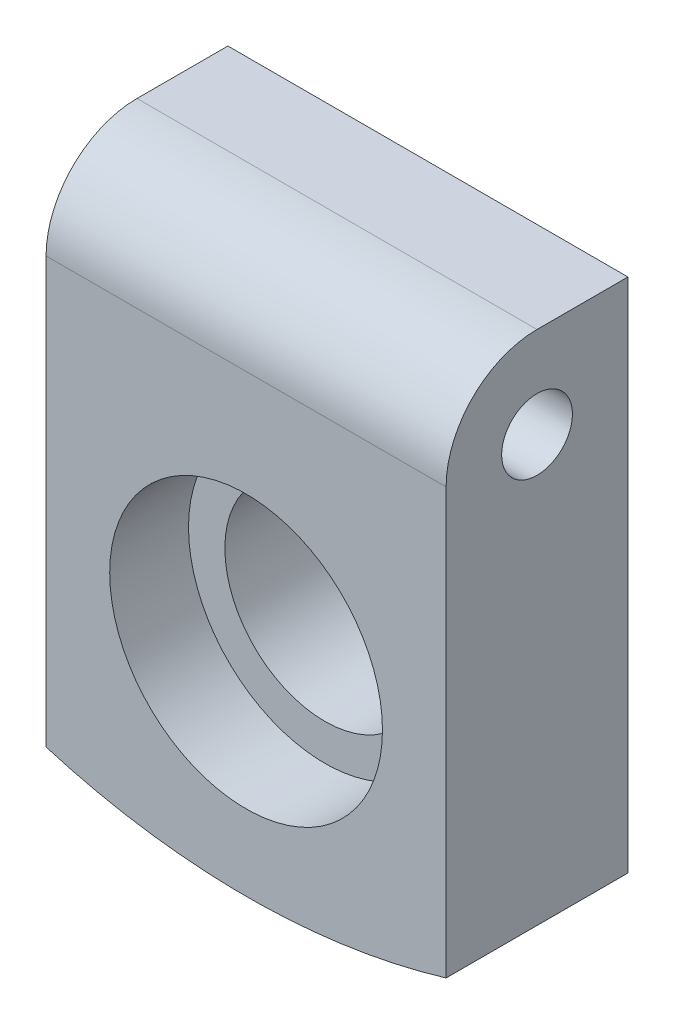
ISO-10303-21;
HEADER;
FILE_DESCRIPTION(('STEP AP214'),'2;1');
FILE_NAME('part.step','',(''),(''),'','','');
FILE_SCHEMA(('AUTOMOTIVE_DESIGN { 1 0 10303 214 1 1 1 1 }'));
ENDSEC;
DATA;
#1=APPLICATION_CONTEXT('core data for automotive mechanical design processes');
#2=APPLICATION_PROTOCOL_DEFINITION('international standard','automotive_design',2000,#1);
#3=PRODUCT_CONTEXT('',#1,'mechanical');
#4=PRODUCT('Part','Part','',(#3));
#5=PRODUCT_RELATED_PRODUCT_CATEGORY('part','',(#4));
#6=PRODUCT_DEFINITION_FORMATION('','',#4);
#7=PRODUCT_DEFINITION_CONTEXT('part definition',#1,'design');
#8=PRODUCT_DEFINITION('design','',#6,#7);
#9=PRODUCT_DEFINITION_SHAPE('','',#8);
#10=(LENGTH_UNIT() NAMED_UNIT(*) SI_UNIT(.MILLI.,.METRE.));
#11=(NAMED_UNIT(*) PLANE_ANGLE_UNIT() SI_UNIT($,.RADIAN.));
#12=(NAMED_UNIT(*) SI_UNIT($,.STERADIAN.) SOLID_ANGLE_UNIT());
#13=UNCERTAINTY_MEASURE_WITH_UNIT(LENGTH_MEASURE(1.E-05),#10,'distance_accuracy_value','');
#14=(GEOMETRIC_REPRESENTATION_CONTEXT(3) GLOBAL_UNCERTAINTY_ASSIGNED_CONTEXT((#13)) GLOBAL_UNIT_ASSIGNED_CONTEXT((#10,
#11,#12)) REPRESENTATION_CONTEXT('',''));
#15=CARTESIAN_POINT('',(0.,0.,0.));
#16=DIRECTION('',(0.,0.,1.));
#17=DIRECTION('',(1.,0.,0.));
#18=AXIS2_PLACEMENT_3D('',#15,#16,#17);
#19=CARTESIAN_POINT('',(0.,0.,15.));
#20=DIRECTION('',(0.,0.,-1.));
#21=DIRECTION('',(-1.,0.,0.));
#22=AXIS2_PLACEMENT_3D('',#19,#20,#21);
#23=PLANE('',#22);
#24=CARTESIAN_POINT('',(0.,-10.,15.));
#25=DIRECTION('',(0.,0.,1.));
#26=DIRECTION('',(1.,0.,0.));
#27=AXIS2_PLACEMENT_3D('',#24,#25,#26);
#28=CIRCLE('',#27,22.5);
#29=CARTESIAN_POINT('',(22.5,-10.,15.));
#30=VERTEX_POINT('',#29);
#31=EDGE_CURVE('E135',#30,#30,#28,.T.);
#32=ORIENTED_EDGE('',*,*,#31,.F.);
#33=EDGE_LOOP('',(#32));
#34=FACE_BOUND('',#33,.T.);
#35=CARTESIAN_POINT('',(0.,70.,15.));
#36=DIRECTION('',(0.,0.,1.));
#37=DIRECTION('',(1.,0.,0.));
#38=AXIS2_PLACEMENT_3D('',#35,#36,#37);
#39=CIRCLE('',#38,115.);
#40=CARTESIAN_POINT('',(-33.,-40.1635148313633,15.));
#41=VERTEX_POINT('',#40);
#42=CARTESIAN_POINT('',(33.,-40.1635148313633,15.));
#43=VERTEX_POINT('',#42);
#44=EDGE_CURVE('E120',#41,#43,#39,.T.);
#45=ORIENTED_EDGE('',*,*,#44,.T.);
#46=DIRECTION('',(0.,1.,0.));
#47=VECTOR('',#46,1.);
#48=CARTESIAN_POINT('',(33.,-45.,15.));
#49=LINE('',#48,#47);
#50=CARTESIAN_POINT('',(33.,30.,15.));
#51=VERTEX_POINT('',#50);
#52=EDGE_CURVE('E124',#43,#51,#49,.T.);
#53=ORIENTED_EDGE('',*,*,#52,.T.);
#54=DIRECTION('',(-1.,0.,0.));
#55=VECTOR('',#54,1.);
#56=CARTESIAN_POINT('',(0.,30.,15.));
#57=LINE('',#56,#55);
#58=CARTESIAN_POINT('',(-33.,30.,15.));
#59=VERTEX_POINT('',#58);
#60=EDGE_CURVE('E143',#51,#59,#57,.T.);
#61=ORIENTED_EDGE('',*,*,#60,.T.);
#62=DIRECTION('',(0.,-1.,0.));
#63=VECTOR('',#62,1.);
#64=CARTESIAN_POINT('',(-33.,-45.,15.));
#65=LINE('',#64,#63);
#66=EDGE_CURVE('E139',#59,#41,#65,.T.);
#67=ORIENTED_EDGE('',*,*,#66,.T.);
#68=EDGE_LOOP('',(#45,#53,#61,#67));
#69=FACE_BOUND('',#68,.T.);
#70=ADVANCED_FACE('F56',(#34,#69),#23,.F.);
#71=CARTESIAN_POINT('',(0.,0.,-15.));
#72=DIRECTION('',(0.,0.,-1.));
#73=DIRECTION('',(-1.,0.,0.));
#74=AXIS2_PLACEMENT_3D('',#71,#72,#73);
#75=PLANE('',#74);
#76=CARTESIAN_POINT('',(0.,-10.,-15.));
#77=DIRECTION('',(0.,0.,-1.));
#78=DIRECTION('',(-1.,0.,0.));
#79=AXIS2_PLACEMENT_3D('',#76,#77,#78);
#80=CIRCLE('',#79,16.5);
#81=CARTESIAN_POINT('',(-16.5,-10.,-15.));
#82=VERTEX_POINT('',#81);
#83=EDGE_CURVE('E208',#82,#82,#80,.T.);
#84=ORIENTED_EDGE('',*,*,#83,.F.);
#85=EDGE_LOOP('',(#84));
#86=FACE_BOUND('',#85,.T.);
#87=DIRECTION('',(0.,1.,0.));
#88=VECTOR('',#87,1.);
#89=CARTESIAN_POINT('',(33.,-45.,-15.));
#90=LINE('',#89,#88);
#91=CARTESIAN_POINT('',(33.,-40.1635148313633,-15.));
#92=VERTEX_POINT('',#91);
#93=CARTESIAN_POINT('',(33.,45.,-15.));
#94=VERTEX_POINT('',#93);
#95=EDGE_CURVE('E122',#92,#94,#90,.T.);
#96=ORIENTED_EDGE('',*,*,#95,.F.);
#97=CARTESIAN_POINT('',(0.,70.,-15.));
#98=DIRECTION('',(0.,0.,1.));
#99=DIRECTION('',(1.,0.,0.));
#100=AXIS2_PLACEMENT_3D('',#97,#98,#99);
#101=CIRCLE('',#100,115.);
#102=CARTESIAN_POINT('',(-33.,-40.1635148313633,-15.));
#103=VERTEX_POINT('',#102);
#104=EDGE_CURVE('E108',#103,#92,#101,.T.);
#105=ORIENTED_EDGE('',*,*,#104,.F.);
#106=DIRECTION('',(0.,-1.,0.));
#107=VECTOR('',#106,1.);
#108=CARTESIAN_POINT('',(-33.,-45.,-15.));
#109=LINE('',#108,#107);
#110=CARTESIAN_POINT('',(-33.,45.,-15.));
#111=VERTEX_POINT('',#110);
#112=EDGE_CURVE('E133',#111,#103,#109,.T.);
#113=ORIENTED_EDGE('',*,*,#112,.F.);
#114=DIRECTION('',(-1.,0.,0.));
#115=VECTOR('',#114,1.);
#116=CARTESIAN_POINT('',(-33.,45.,-15.));
#117=LINE('',#116,#115);
#118=EDGE_CURVE('E129',#94,#111,#117,.T.);
#119=ORIENTED_EDGE('',*,*,#118,.F.);
#120=EDGE_LOOP('',(#96,#105,#113,#119));
#121=FACE_BOUND('',#120,.T.);
#122=ADVANCED_FACE('F127',(#86,#121),#75,.T.);
#123=CARTESIAN_POINT('',(33.,-45.,15.));
#124=DIRECTION('',(-1.,0.,0.));
#125=DIRECTION('',(0.,0.,1.));
#126=AXIS2_PLACEMENT_3D('',#123,#124,#125);
#127=PLANE('',#126);
#128=CARTESIAN_POINT('',(33.,30.,0.));
#129=DIRECTION('',(-1.,0.,0.));
#130=DIRECTION('',(0.,0.,1.));
#131=AXIS2_PLACEMENT_3D('',#128,#129,#130);
#132=CIRCLE('',#131,5.83992937773841);
#133=CARTESIAN_POINT('',(33.,30.,5.83992937773841));
#134=VERTEX_POINT('',#133);
#135=EDGE_CURVE('E64',#134,#134,#132,.T.);
#136=ORIENTED_EDGE('',*,*,#135,.T.);
#137=EDGE_LOOP('',(#136));
#138=FACE_BOUND('',#137,.T.);
#139=DIRECTION('',(0.,0.,1.));
#140=VECTOR('',#139,1.);
#141=CARTESIAN_POINT('',(33.,-40.1635148313633,-15.));
#142=LINE('',#141,#140);
#143=EDGE_CURVE('E111',#92,#43,#142,.T.);
#144=ORIENTED_EDGE('',*,*,#143,.F.);
#145=ORIENTED_EDGE('',*,*,#95,.T.);
#146=DIRECTION('',(0.,0.,-1.));
#147=VECTOR('',#146,1.);
#148=CARTESIAN_POINT('',(33.,45.,15.));
#149=LINE('',#148,#147);
#150=CARTESIAN_POINT('',(33.,45.,0.));
#151=VERTEX_POINT('',#150);
#152=EDGE_CURVE('E141',#151,#94,#149,.T.);
#153=ORIENTED_EDGE('',*,*,#152,.F.);
#154=CARTESIAN_POINT('',(33.,30.,0.));
#155=DIRECTION('',(-1.,0.,0.));
#156=DIRECTION('',(0.,0.,1.));
#157=AXIS2_PLACEMENT_3D('',#154,#155,#156);
#158=CIRCLE('',#157,15.);
#159=EDGE_CURVE('E153',#151,#51,#158,.F.);
#160=ORIENTED_EDGE('',*,*,#159,.T.);
#161=ORIENTED_EDGE('',*,*,#52,.F.);
#162=EDGE_LOOP('',(#144,#145,#153,#160,#161));
#163=FACE_BOUND('',#162,.T.);
#164=ADVANCED_FACE('F119',(#138,#163),#127,.F.);
#165=CARTESIAN_POINT('',(-33.,-45.,15.));
#166=DIRECTION('',(1.,0.,0.));
#167=DIRECTION('',(0.,0.,-1.));
#168=AXIS2_PLACEMENT_3D('',#165,#166,#167);
#169=PLANE('',#168);
#170=CARTESIAN_POINT('',(-33.,30.,0.));
#171=DIRECTION('',(1.,0.,0.));
#172=DIRECTION('',(0.,0.,-1.));
#173=AXIS2_PLACEMENT_3D('',#170,#171,#172);
#174=CIRCLE('',#173,6.50199999999991);
#175=CARTESIAN_POINT('',(-33.,30.,-6.50199999999991));
#176=VERTEX_POINT('',#175);
#177=EDGE_CURVE('E12',#176,#176,#174,.T.);
#178=ORIENTED_EDGE('',*,*,#177,.T.);
#179=EDGE_LOOP('',(#178));
#180=FACE_BOUND('',#179,.T.);
#181=DIRECTION('',(0.,0.,1.));
#182=VECTOR('',#181,1.);
#183=CARTESIAN_POINT('',(-33.,-40.1635148313633,-15.));
#184=LINE('',#183,#182);
#185=EDGE_CURVE('E77',#103,#41,#184,.T.);
#186=ORIENTED_EDGE('',*,*,#185,.T.);
#187=ORIENTED_EDGE('',*,*,#66,.F.);
#188=CARTESIAN_POINT('',(-33.,30.,0.));
#189=DIRECTION('',(1.,0.,0.));
#190=DIRECTION('',(0.,0.,-1.));
#191=AXIS2_PLACEMENT_3D('',#188,#189,#190);
#192=CIRCLE('',#191,15.);
#193=CARTESIAN_POINT('',(-33.,45.,0.));
#194=VERTEX_POINT('',#193);
#195=EDGE_CURVE('E149',#59,#194,#192,.F.);
#196=ORIENTED_EDGE('',*,*,#195,.T.);
#197=DIRECTION('',(0.,0.,-1.));
#198=VECTOR('',#197,1.);
#199=CARTESIAN_POINT('',(-33.,45.,15.));
#200=LINE('',#199,#198);
#201=EDGE_CURVE('E142',#194,#111,#200,.T.);
#202=ORIENTED_EDGE('',*,*,#201,.T.);
#203=ORIENTED_EDGE('',*,*,#112,.T.);
#204=EDGE_LOOP('',(#186,#187,#196,#202,#203));
#205=FACE_BOUND('',#204,.T.);
#206=ADVANCED_FACE('F181',(#180,#205),#169,.F.);
#207=CARTESIAN_POINT('',(-33.,45.,15.));
#208=DIRECTION('',(0.,-1.,0.));
#209=DIRECTION('',(0.,0.,-1.));
#210=AXIS2_PLACEMENT_3D('',#207,#208,#209);
#211=PLANE('',#210);
#212=ORIENTED_EDGE('',*,*,#201,.F.);
#213=DIRECTION('',(-1.,0.,0.));
#214=VECTOR('',#213,1.);
#215=CARTESIAN_POINT('',(-33.,45.,0.));
#216=LINE('',#215,#214);
#217=EDGE_CURVE('E81',#194,#151,#216,.F.);
#218=ORIENTED_EDGE('',*,*,#217,.T.);
#219=ORIENTED_EDGE('',*,*,#152,.T.);
#220=ORIENTED_EDGE('',*,*,#118,.T.);
#221=EDGE_LOOP('',(#212,#218,#219,#220));
#222=FACE_BOUND('',#221,.T.);
#223=ADVANCED_FACE('F183',(#222),#211,.F.);
#224=CARTESIAN_POINT('',(0.,-10.,2.));
#225=DIRECTION('',(0.,0.,1.));
#226=DIRECTION('',(1.,0.,0.));
#227=AXIS2_PLACEMENT_3D('',#224,#225,#226);
#228=CYLINDRICAL_SURFACE('',#227,22.5);
#229=CARTESIAN_POINT('',(0.,-10.,2.));
#230=DIRECTION('',(0.,0.,1.));
#231=DIRECTION('',(1.,0.,0.));
#232=AXIS2_PLACEMENT_3D('',#229,#230,#231);
#233=CIRCLE('',#232,22.5);
#234=CARTESIAN_POINT('',(22.5,-10.,2.));
#235=VERTEX_POINT('',#234);
#236=EDGE_CURVE('E126',#235,#235,#233,.T.);
#237=CARTESIAN_POINT('',(22.5,-10.,2.));
#238=CARTESIAN_POINT('',(22.5,-10.,2.13541666666667));
#239=CARTESIAN_POINT('',(22.5,-10.,2.27083333333333));
#240=CARTESIAN_POINT('',(22.5,-10.,2.54166666666667));
#241=CARTESIAN_POINT('',(22.5,-10.,2.67708333333333));
#242=CARTESIAN_POINT('',(22.5,-10.,2.94791666666667));
#243=CARTESIAN_POINT('',(22.5,-10.,3.08333333333333));
#244=CARTESIAN_POINT('',(22.5,-10.,3.35416666666667));
#245=CARTESIAN_POINT('',(22.5,-10.,3.48958333333333));
#246=CARTESIAN_POINT('',(22.5,-10.,3.76041666666667));
#247=CARTESIAN_POINT('',(22.5,-10.,3.89583333333333));
#248=CARTESIAN_POINT('',(22.5,-10.,4.16666666666667));
#249=CARTESIAN_POINT('',(22.5,-10.,4.30208333333333));
#250=CARTESIAN_POINT('',(22.5,-10.,4.57291666666667));
#251=CARTESIAN_POINT('',(22.5,-10.,4.70833333333333));
#252=CARTESIAN_POINT('',(22.5,-10.,4.97916666666667));
#253=CARTESIAN_POINT('',(22.5,-10.,5.11458333333333));
#254=CARTESIAN_POINT('',(22.5,-10.,5.38541666666667));
#255=CARTESIAN_POINT('',(22.5,-10.,5.52083333333333));
#256=CARTESIAN_POINT('',(22.5,-10.,5.79166666666667));
#257=CARTESIAN_POINT('',(22.5,-10.,5.92708333333333));
#258=CARTESIAN_POINT('',(22.5,-10.,6.19791666666667));
#259=CARTESIAN_POINT('',(22.5,-10.,6.33333333333333));
#260=CARTESIAN_POINT('',(22.5,-10.,6.60416666666667));
#261=CARTESIAN_POINT('',(22.5,-10.,6.73958333333333));
#262=CARTESIAN_POINT('',(22.5,-10.,7.01041666666667));
#263=CARTESIAN_POINT('',(22.5,-10.,7.14583333333333));
#264=CARTESIAN_POINT('',(22.5,-10.,7.41666666666667));
#265=CARTESIAN_POINT('',(22.5,-10.,7.55208333333333));
#266=CARTESIAN_POINT('',(22.5,-10.,7.82291666666667));
#267=CARTESIAN_POINT('',(22.5,-10.,7.95833333333333));
#268=CARTESIAN_POINT('',(22.5,-10.,8.22916666666667));
#269=CARTESIAN_POINT('',(22.5,-10.,8.36458333333333));
#270=CARTESIAN_POINT('',(22.5,-10.,8.63541666666667));
#271=CARTESIAN_POINT('',(22.5,-10.,8.77083333333333));
#272=CARTESIAN_POINT('',(22.5,-10.,9.04166666666667));
#273=CARTESIAN_POINT('',(22.5,-10.,9.17708333333333));
#274=CARTESIAN_POINT('',(22.5,-10.,9.44791666666667));
#275=CARTESIAN_POINT('',(22.5,-10.,9.58333333333333));
#276=CARTESIAN_POINT('',(22.5,-10.,9.85416666666667));
#277=CARTESIAN_POINT('',(22.5,-10.,9.98958333333333));
#278=CARTESIAN_POINT('',(22.5,-10.,10.2604166666667));
#279=CARTESIAN_POINT('',(22.5,-10.,10.3958333333333));
#280=CARTESIAN_POINT('',(22.5,-10.,10.6666666666667));
#281=CARTESIAN_POINT('',(22.5,-10.,10.8020833333333));
#282=CARTESIAN_POINT('',(22.5,-10.,11.0729166666667));
#283=CARTESIAN_POINT('',(22.5,-10.,11.2083333333333));
#284=CARTESIAN_POINT('',(22.5,-10.,11.4791666666667));
#285=CARTESIAN_POINT('',(22.5,-10.,11.6145833333333));
#286=CARTESIAN_POINT('',(22.5,-10.,11.8854166666667));
#287=CARTESIAN_POINT('',(22.5,-10.,12.0208333333333));
#288=CARTESIAN_POINT('',(22.5,-10.,12.2916666666667));
#289=CARTESIAN_POINT('',(22.5,-10.,12.4270833333333));
#290=CARTESIAN_POINT('',(22.5,-10.,12.6979166666667));
#291=CARTESIAN_POINT('',(22.5,-10.,12.8333333333333));
#292=CARTESIAN_POINT('',(22.5,-10.,13.1041666666667));
#293=CARTESIAN_POINT('',(22.5,-10.,13.2395833333333));
#294=CARTESIAN_POINT('',(22.5,-10.,13.5104166666667));
#295=CARTESIAN_POINT('',(22.5,-10.,13.6458333333333));
#296=CARTESIAN_POINT('',(22.5,-10.,13.9166666666667));
#297=CARTESIAN_POINT('',(22.5,-10.,14.0520833333333));
#298=CARTESIAN_POINT('',(22.5,-10.,14.3229166666667));
#299=CARTESIAN_POINT('',(22.5,-10.,14.4583333333333));
#300=CARTESIAN_POINT('',(22.5,-10.,14.7291666666667));
#301=CARTESIAN_POINT('',(22.5,-10.,14.8645833333333));
#302=CARTESIAN_POINT('',(22.5,-10.,15.));
#303=B_SPLINE_CURVE_WITH_KNOTS('',3,(#237,#238,#239,#240,#241,#242,#243,#244,#245,#246,#247,
#248,#249,#250,#251,#252,#253,#254,#255,#256,#257,#258,#259,#260,#261,#262,#263,#264,#265,#266,
#267,#268,#269,#270,#271,#272,#273,#274,#275,#276,#277,#278,#279,#280,#281,#282,#283,#284,#285,
#286,#287,#288,#289,#290,#291,#292,#293,#294,#295,#296,#297,#298,#299,#300,#301,#302),
.UNSPECIFIED.,.F.,.F.,(4,2,2,2,2,2,2,2,2,2,2,2,2,2,2,2,2,2,2,2,2,2,2,2,2,2,2,2,2,2,2,2,4),(0.,
0.40625,0.8125,1.21875,1.625,2.03125,2.4375,2.84375,3.25,3.65625,4.0625,4.46875,4.875,5.28125,
5.6875,6.09375,6.5,6.90625,7.3125,7.71875,8.125,8.53125,8.9375,9.34375,9.75,10.15625,10.5625,
10.96875,11.375,11.78125,12.1875,12.59375,13.),.UNSPECIFIED.);
#304=EDGE_CURVE('BSEAM178',#235,#30,#303,.T.);
#305=ORIENTED_EDGE('',*,*,#236,.F.);
#306=ORIENTED_EDGE('',*,*,#31,.T.);
#307=ORIENTED_EDGE('',*,*,#304,.T.);
#308=ORIENTED_EDGE('',*,*,#304,.F.);
#309=EDGE_LOOP('',(#305,#307,#306,#308));
#310=FACE_BOUND('',#309,.T.);
#311=ADVANCED_FACE('F178',(#310),#228,.F.);
#312=CARTESIAN_POINT('',(0.,-10.,2.));
#313=DIRECTION('',(0.,0.,1.));
#314=DIRECTION('',(1.,0.,0.));
#315=AXIS2_PLACEMENT_3D('',#312,#313,#314);
#316=PLANE('',#315);
#317=CARTESIAN_POINT('',(0.,-10.,2.));
#318=DIRECTION('',(0.,0.,-1.));
#319=DIRECTION('',(-1.,0.,0.));
#320=AXIS2_PLACEMENT_3D('',#317,#318,#319);
#321=CIRCLE('',#320,16.5);
#322=CARTESIAN_POINT('',(-16.5,-10.,2.));
#323=VERTEX_POINT('',#322);
#324=EDGE_CURVE('E206',#323,#323,#321,.T.);
#325=ORIENTED_EDGE('',*,*,#324,.T.);
#326=EDGE_LOOP('',(#325));
#327=FACE_BOUND('',#326,.T.);
#328=ORIENTED_EDGE('',*,*,#236,.T.);
#329=EDGE_LOOP('',(#328));
#330=FACE_BOUND('',#329,.T.);
#331=ADVANCED_FACE('F197',(#327,#330),#316,.T.);
#332=CARTESIAN_POINT('',(0.,-10.,2.));
#333=DIRECTION('',(0.,0.,-1.));
#334=DIRECTION('',(-1.,0.,0.));
#335=AXIS2_PLACEMENT_3D('',#332,#333,#334);
#336=CYLINDRICAL_SURFACE('',#335,16.5);
#337=ORIENTED_EDGE('',*,*,#324,.F.);
#338=EDGE_LOOP('',(#337));
#339=FACE_BOUND('',#338,.T.);
#340=ORIENTED_EDGE('',*,*,#83,.T.);
#341=EDGE_LOOP('',(#340));
#342=FACE_BOUND('',#341,.T.);
#343=ADVANCED_FACE('F192',(#339,#342),#336,.F.);
#344=CARTESIAN_POINT('',(0.,30.,0.));
#345=DIRECTION('',(-1.,0.,0.));
#346=DIRECTION('',(0.,0.,1.));
#347=AXIS2_PLACEMENT_3D('',#344,#345,#346);
#348=CYLINDRICAL_SURFACE('',#347,15.);
#349=ORIENTED_EDGE('',*,*,#159,.F.);
#350=ORIENTED_EDGE('',*,*,#217,.F.);
#351=ORIENTED_EDGE('',*,*,#195,.F.);
#352=ORIENTED_EDGE('',*,*,#60,.F.);
#353=EDGE_LOOP('',(#349,#350,#351,#352));
#354=FACE_BOUND('',#353,.T.);
#355=ADVANCED_FACE('F188',(#354),#348,.T.);
#356=CARTESIAN_POINT('',(0.,70.,-15.));
#357=DIRECTION('',(0.,0.,1.));
#358=DIRECTION('',(1.,0.,0.));
#359=AXIS2_PLACEMENT_3D('',#356,#357,#358);
#360=CYLINDRICAL_SURFACE('',#359,115.);
#361=ORIENTED_EDGE('',*,*,#44,.F.);
#362=ORIENTED_EDGE('',*,*,#185,.F.);
#363=ORIENTED_EDGE('',*,*,#104,.T.);
#364=ORIENTED_EDGE('',*,*,#143,.T.);
#365=EDGE_LOOP('',(#361,#362,#363,#364));
#366=FACE_BOUND('',#365,.T.);
#367=ADVANCED_FACE('F109',(#366),#360,.T.);
#368=CARTESIAN_POINT('',(-33.,30.,0.));
#369=DIRECTION('',(-1.,0.,0.));
#370=DIRECTION('',(0.,0.,1.));
#371=AXIS2_PLACEMENT_3D('',#368,#369,#370);
#372=CONICAL_SURFACE('',#371,6.5,0.0100007366139275);
#373=CARTESIAN_POINT('',(-32.9999799958591,30.,0.));
#374=DIRECTION('',(1.,0.,0.));
#375=DIRECTION('',(0.,0.,-1.));
#376=AXIS2_PLACEMENT_3D('',#373,#374,#375);
#377=CIRCLE('',#376,6.49999979993719);
#378=CARTESIAN_POINT('',(-32.9999799958591,30.,-6.49999979993719));
#379=VERTEX_POINT('',#378);
#380=EDGE_CURVE('E67',#379,#379,#377,.F.);
#381=ORIENTED_EDGE('',*,*,#380,.T.);
#382=EDGE_LOOP('',(#381));
#383=FACE_BOUND('',#382,.T.);
#384=ORIENTED_EDGE('',*,*,#135,.F.);
#385=EDGE_LOOP('',(#384));
#386=FACE_BOUND('',#385,.T.);
#387=ADVANCED_FACE('F62',(#383,#386),#372,.F.);
#388=CARTESIAN_POINT('',(-32.9999799978599,30.,0.));
#389=DIRECTION('',(-1.,0.,0.));
#390=DIRECTION('',(0.,0.,1.));
#391=AXIS2_PLACEMENT_3D('',#388,#389,#390);
#392=CONICAL_SURFACE('',#391,6.5,1.56079559018016);
#393=ORIENTED_EDGE('',*,*,#177,.F.);
#394=EDGE_LOOP('',(#393));
#395=FACE_BOUND('',#394,.T.);
#396=ORIENTED_EDGE('',*,*,#380,.F.);
#397=EDGE_LOOP('',(#396));
#398=FACE_BOUND('',#397,.T.);
#399=ADVANCED_FACE('F159',(#395,#398),#392,.F.);
#400=CLOSED_SHELL('',(#70,#122,#164,#206,#223,#311,#331,#343,#355,#367,#387,#399));
#401=MANIFOLD_SOLID_BREP('B2',#400);
#402=ADVANCED_BREP_SHAPE_REPRESENTATION('',(#18,#401),#14);
#403=SHAPE_DEFINITION_REPRESENTATION(#9,#402);
ENDSEC;
END-ISO-10303-21;
